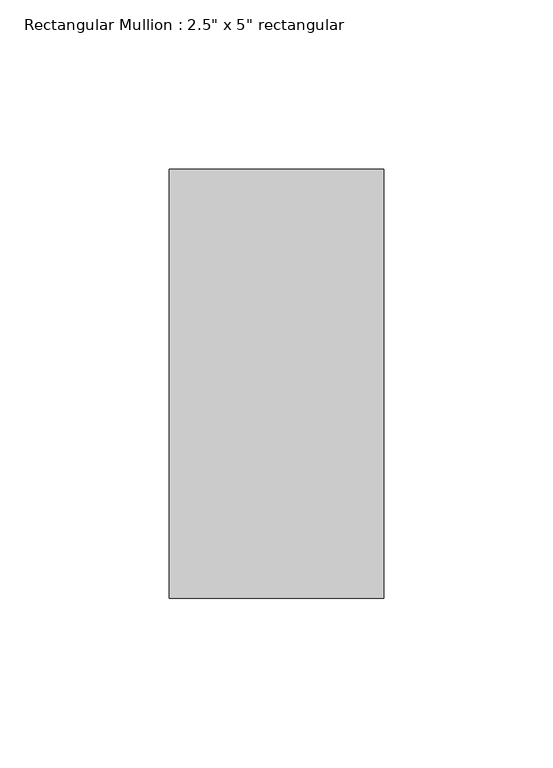
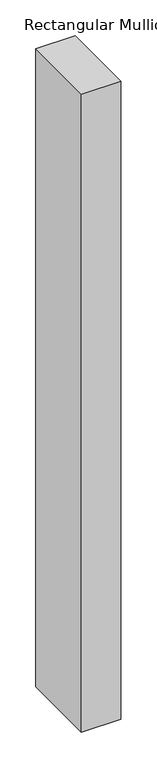
"""IFC4 building model written with IfcOpenShell, lengths in millimetres: member geometry."""

from ifc_helpers import new_model, si_unit, frame, origin, place, context, project, spatial, polyline, outline, extrude, source, transform, mapped, element, save


def member_0cc0e230(model_context):
    return source(origin(), model_context, "Body", "SweptSolid", [
        extrude(outline(polyline([(31.75, 63.5), (31.75, -63.5), (-31.75, -63.5), (-31.75, 63.5), (31.75, 63.5)])), frame((0.0, 0.0, -1085.8500002), z_axis=(0.0, 0.0, 1.0), x_axis=(1.0, 0.0, 0.0)), (0.0, 0.0, 1.0), 1085.8500002),
    ])


if __name__ == "__main__":
    model = new_model("IFC4")
    model_context = context("Model", 3, world=origin())
    ifc_project = project(units=[si_unit("LENGTHUNIT", "METRE", prefix="MILLI")], contexts=[model_context])
    site = spatial("IfcSite", under=ifc_project)
    building = spatial("IfcBuilding", under=site)
    placement = place(None, origin())
    member_shape = member_0cc0e230(model_context)
    element("IfcMember", 1, ObjectType="Rectangular Mullion : 2.5\" x 5\" rectangular", at=placement, inside=building, context=model_context, shape_type="MappedRepresentation", body=[
        mapped(member_shape, transform((0.0, 0.0, 0.0), x_axis=(1.0, 0.0, 0.0), y_axis=(0.0, 1.0, 0.0), z_axis=(0.0, 0.0, 1.0))),
    ])
    save(model, "model.ifc")

# Revit data of these elements
# Type "Rectangular Mullion : 2.5\" x 5\" rectangular"
#   built-in parameter 1007304 = 0.416667 (stored number, unit not read)
#   built-in parameter 1007301 = 0.104167 (stored number, unit not read)
#   built-in parameter 1007300 = 0.104167 (stored number, unit not read)
# Element 1 (IfcMember, "Rectangular Mullion : 2.5\" x 5\" rectangular")
#   Materials on its faces: "Aluminum"
# Materials
#   "Aluminum": class "Metal", colour RGB 247 247 247, transparency 0, Description = "Aluminum 6061", Cost = 0
